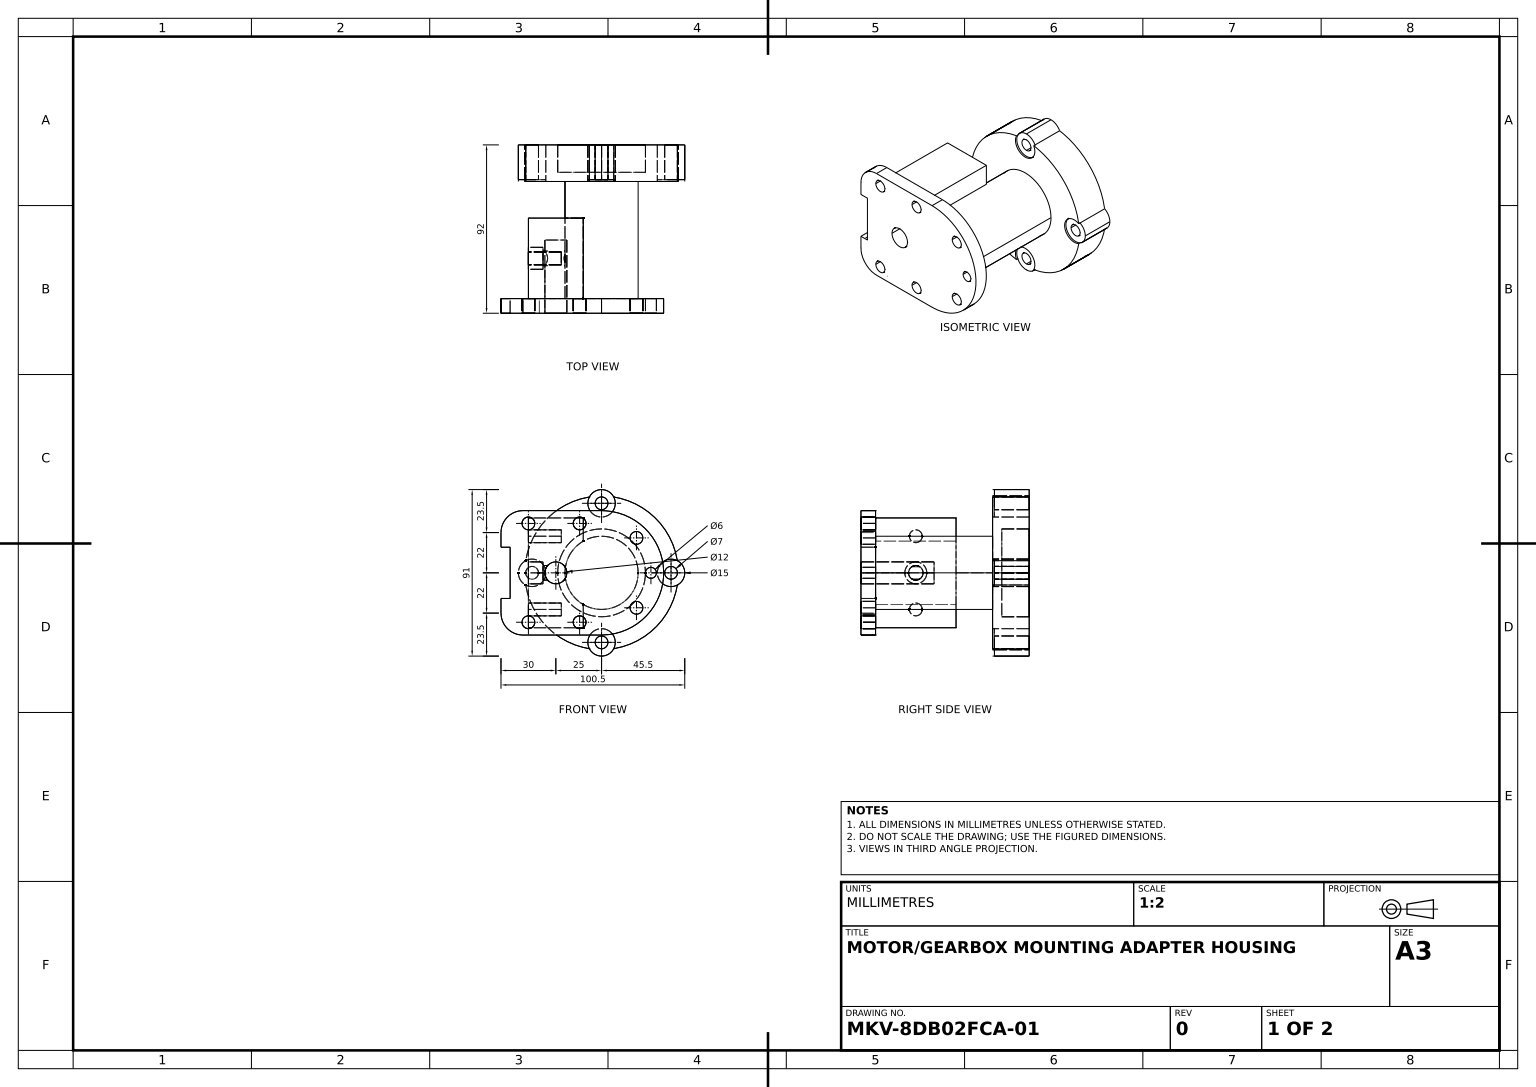
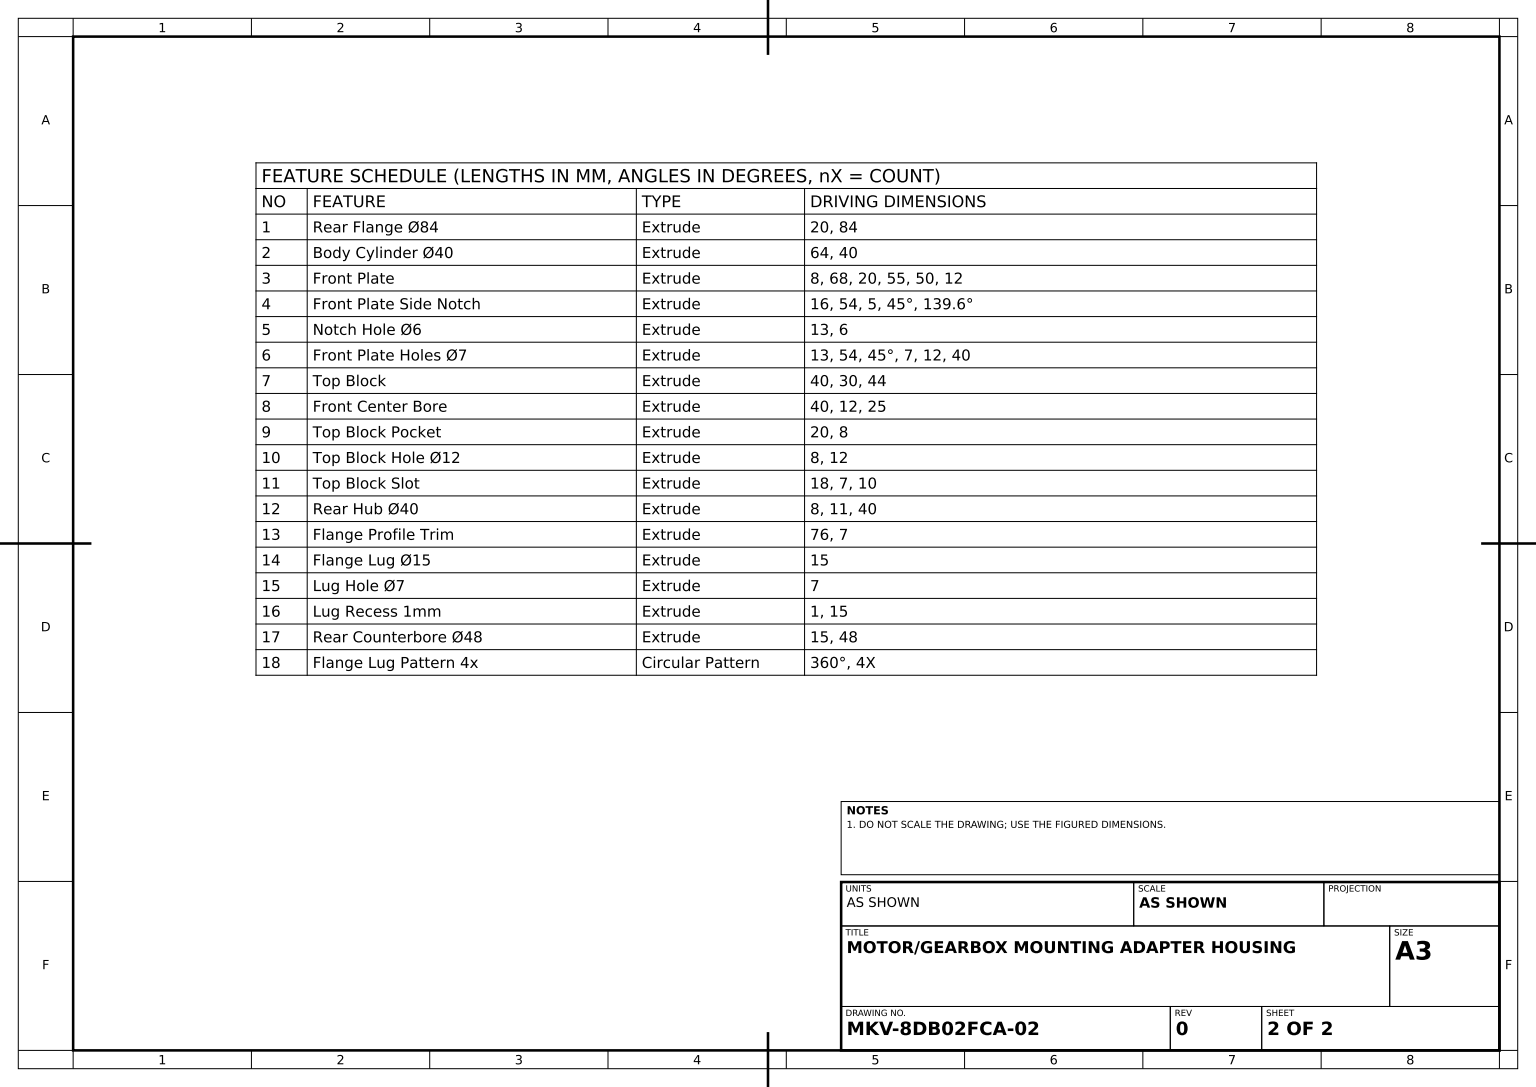
from build123d import *

# Parameters (mm, degrees)
REAR_FLANGE_SKETCH_84_R         = 42
REAR_FLANGE_84_DEPTH            = 20
BODY_CYLINDER_SKETCH_40_R       = 20
BODY_CYLINDER_40_DEPTH          = 64
FRONT_PLATE_DEPTH               = 8
FRONT_PLATE_SIDE_NOTCH_SKETCH_R = 2.5
FRONT_PLATE_SIDE_NOTCH_DEPTH    = 16
NOTCH_HOLE_SKETCH_6_R           = 3
NOTCH_HOLE_6_DEPTH              = 13
FRONT_PLATE_HOLES_SKETCH_R      = 3.5
FRONT_PLATE_HOLES_7_DEPTH       = 13
TOP_BLOCK_DEPTH                 = 30
FRONT_CENTER_BORE_SKETCH_R      = 6
FRONT_CENTER_BORE_DEPTH         = 40
TOP_BLOCK_POCKET_SKETCH_R       = 4
TOP_BLOCK_POCKET_DEPTH          = 20
TOP_BLOCK_HOLE_SKETCH_12_R      = 6
TOP_BLOCK_HOLE_12_DEPTH         = 8
TOP_BLOCK_SLOT_SKETCH_R         = 3.5
TOP_BLOCK_SLOT_DEPTH            = 18
REAR_HUB_SKETCH_40_R            = 20
REAR_HUB_40_DEPTH               = 11
FLANGE_PROFILE_TRIM_SKETCH_R    = 3.5
FLANGE_PROFILE_TRIM_DEPTH       = 100.864908824
FLANGE_LUG_SKETCH_15_R          = 7.5
FLANGE_LUG_15_DEPTH             = 20
LUG_HOLE_SKETCH_7_R             = 3.5
LUG_HOLE_7_DEPTH                = 100.864908824
LUG_RECESS_SKETCH_R             = 7.5
LUG_RECESS_1MM_DEPTH            = 1
REAR_COUNTERBORE_SKETCH_48_R    = 24
REAR_COUNTERBORE_48_DEPTH       = 15
FLANGE_LUG_PATTERN_4X_COUNT     = 4


with BuildPart() as part:
    # Rear Flange Sketch Ø84 → Rear Flange Ø84 (new body)
    with BuildSketch(Plane.XY):
        Circle(REAR_FLANGE_SKETCH_84_R)
    extrude(amount=REAR_FLANGE_84_DEPTH)

    # Body Cylinder Sketch Ø40 → Body Cylinder Ø40 (add)
    with BuildSketch(Plane.XY.offset(20)):
        Circle(BODY_CYLINDER_SKETCH_40_R)
    extrude(amount=BODY_CYLINDER_40_DEPTH)

    # Front Plate Sketch → Front Plate (add)
    with BuildSketch(Plane.XY.offset(84)):
        with BuildLine():
            Line((0, 34), (-43, 34))
            ThreePointArc((-43, 34), (-51.485281374, 30.485281374), (-55, 22))
            Line((-55, 22), (-55, 14))
            Line((-55, 14), (-50, 14))
            Line((-50, 14), (-50, 0))
            Line((-50, 0), (-50, -14))
            Line((-50, -14), (-55, -14))
            Line((-55, -14), (-55, -22))
            ThreePointArc((-55, -22), (-51.485281374, -30.485281374), (-43, -34))
            Line((-43, -34), (0, -34))
            ThreePointArc((0, -34), (34, 0), (0, 34))
        make_face()
    extrude(amount=FRONT_PLATE_DEPTH)

    # Front Plate Side Notch Sketch → Front Plate Side Notch (cut)
    with BuildSketch(Plane.XY.offset(92)):
        with Locations((27, 0)):
            Circle(FRONT_PLATE_SIDE_NOTCH_SKETCH_R)
    extrude(amount=-FRONT_PLATE_SIDE_NOTCH_DEPTH, mode=Mode.SUBTRACT)

    # Notch Hole Sketch Ø6 → Notch Hole Ø6 (cut)
    with BuildSketch(Plane.XY.offset(92)):
        with Locations((27, 0)):
            Circle(NOTCH_HOLE_SKETCH_6_R)
    extrude(amount=-NOTCH_HOLE_6_DEPTH, mode=Mode.SUBTRACT)

    # Front Plate Holes Sketch → Front Plate Holes Ø7 (cut)
    with BuildSketch(Plane.XY.offset(92)):
        with Locations((19.091883092, 19.091883092)):
            Circle(FRONT_PLATE_HOLES_SKETCH_R)
        with Locations((19.091883092, -19.091883092)):
            Circle(FRONT_PLATE_HOLES_SKETCH_R)
        with Locations((-12, 27)):
            Circle(FRONT_PLATE_HOLES_SKETCH_R)
        with Locations((-40, 27)):
            Circle(FRONT_PLATE_HOLES_SKETCH_R)
        with Locations((-12, -27)):
            Circle(FRONT_PLATE_HOLES_SKETCH_R)
        with Locations((-40, -27)):
            Circle(FRONT_PLATE_HOLES_SKETCH_R)
    extrude(amount=-FRONT_PLATE_HOLES_7_DEPTH, mode=Mode.SUBTRACT)

    # Top Block Sketch → Top Block (add)
    with BuildSketch(Plane(origin=(-40, 0, 0), x_dir=(0, 0, -1), z_dir=(1, 0, 0))):
        Polygon((-84, 30), (-84, 0), (-84, -30), (-40, -30), (-40, 0), (-40, 30), align=None)
    extrude(amount=TOP_BLOCK_DEPTH)

    # Front Center Bore Sketch → Front Center Bore (cut)
    with BuildSketch(Plane.XY.offset(92)):
        with Locations((-25, 0)):
            Circle(FRONT_CENTER_BORE_SKETCH_R)
    extrude(amount=-FRONT_CENTER_BORE_DEPTH, mode=Mode.SUBTRACT)

    # Top Block Pocket Sketch → Top Block Pocket (cut)
    with BuildSketch(Plane.ZY.offset(40)):
        with Locations((62, 0)):
            Circle(TOP_BLOCK_POCKET_SKETCH_R)
    extrude(amount=-TOP_BLOCK_POCKET_DEPTH, mode=Mode.SUBTRACT)

    # Top Block Hole Sketch Ø12 → Top Block Hole Ø12 (cut)
    with BuildSketch(Plane.ZY.offset(40)):
        with Locations((62, 0)):
            Circle(TOP_BLOCK_HOLE_SKETCH_12_R)
    extrude(amount=-TOP_BLOCK_HOLE_12_DEPTH, mode=Mode.SUBTRACT)

    # Top Block Slot Sketch → Top Block Slot (cut)
    with BuildSketch(Plane.ZY.offset(40)):
        with Locations((62, 20)):
            Circle(TOP_BLOCK_SLOT_SKETCH_R)
        with Locations((62, -20)):
            Circle(TOP_BLOCK_SLOT_SKETCH_R)
    extrude(amount=-TOP_BLOCK_SLOT_DEPTH, mode=Mode.SUBTRACT)

    # Rear Hub Sketch Ø40 → Rear Hub Ø40 (add)
    with BuildSketch(Plane.XY.offset(8)):
        with Locations(Location((0, 0, 0), (0, 0, 240))):
            Circle(REAR_HUB_SKETCH_40_R)
    extrude(amount=REAR_HUB_40_DEPTH)

    # Flange Profile Trim Sketch → Flange Profile Trim (cut, through all)
    with BuildSketch(Plane.XY.offset(20)):
        with Locations((38, 0)):
            Circle(FLANGE_PROFILE_TRIM_SKETCH_R)
    extrude(amount=-FLANGE_PROFILE_TRIM_DEPTH, mode=Mode.SUBTRACT)

    # Flange Lug Sketch Ø15 → Flange Lug Ø15 (add, through all)
    with BuildSketch(Plane.XY.offset(20)):
        with Locations((38, 0)):
            Circle(FLANGE_LUG_SKETCH_15_R)
    flange_lug_15 = extrude(amount=-FLANGE_LUG_15_DEPTH)

    # Lug Hole Sketch Ø7 → Lug Hole Ø7 (cut, through all)
    with BuildSketch(Plane.XY.offset(20)):
        with Locations((38, 0)):
            Circle(LUG_HOLE_SKETCH_7_R)
    lug_hole_7 = extrude(amount=-LUG_HOLE_7_DEPTH, mode=Mode.SUBTRACT)

    # Lug Recess Sketch → Lug Recess 1mm (cut)
    with BuildSketch(Plane.XY.offset(20)):
        with Locations((38, 0)):
            Circle(LUG_RECESS_SKETCH_R)
    lug_recess_1mm = extrude(amount=-LUG_RECESS_1MM_DEPTH, mode=Mode.SUBTRACT)

    # Rear Counterbore Sketch Ø48 → Rear Counterbore Ø48 (cut)
    with BuildSketch(Plane(origin=(0, 0, 0), x_dir=(-1, 0, 0), z_dir=(0, 0, -1))):
        Circle(REAR_COUNTERBORE_SKETCH_48_R)
    extrude(amount=-REAR_COUNTERBORE_48_DEPTH, mode=Mode.SUBTRACT)

    # Flange Lug Pattern 4x: Flange Lug Ø15, Lug Hole Ø7, Lug Recess 1mm ×4 about axis
    flange_lug_pattern_4x_axis = Axis((0, 0, 0), (0, 0, 1))
    add([flange_lug_15.rotate(flange_lug_pattern_4x_axis, i * 360 / FLANGE_LUG_PATTERN_4X_COUNT) for i in range(1, FLANGE_LUG_PATTERN_4X_COUNT)])
    add([lug_hole_7.rotate(flange_lug_pattern_4x_axis, i * 360 / FLANGE_LUG_PATTERN_4X_COUNT) for i in range(1, FLANGE_LUG_PATTERN_4X_COUNT)], mode=Mode.SUBTRACT)
    add([lug_recess_1mm.rotate(flange_lug_pattern_4x_axis, i * 360 / FLANGE_LUG_PATTERN_4X_COUNT) for i in range(1, FLANGE_LUG_PATTERN_4X_COUNT)], mode=Mode.SUBTRACT)


solid = part.part
